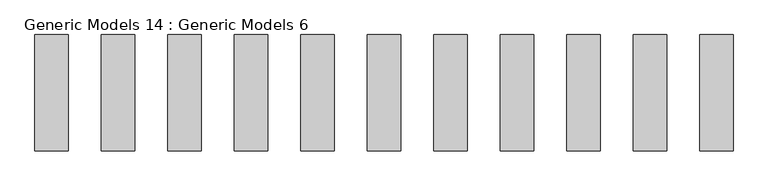
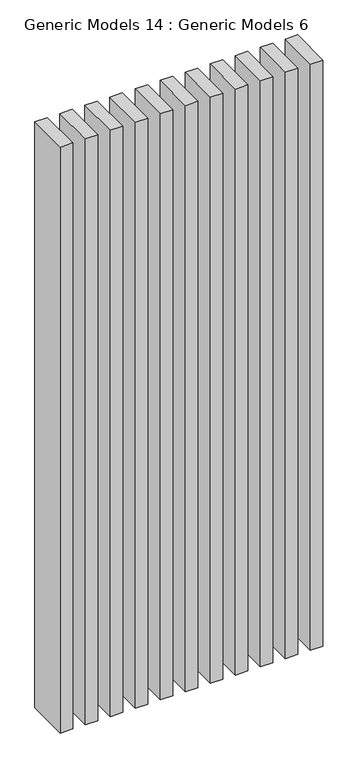
"""IFC4 building model written with IfcOpenShell, lengths in millimetres: proxy geometry, Generic Models 14 : Generic Models 6."""

from ifc_helpers import new_model, si_unit, frame, origin, place, context, project, spatial, polyline, outline, extrude, source, transform, mapped, element, save


def generic_models_14_generic_models_6_3cb9ea36(model_context):
    return source(origin(), model_context, "Body", "SweptSolid", [
        extrude(outline(polyline([(-7087.8263252, -11102.5719459), (-7138.6263252, -11102.5719459), (-7138.6263252, -10924.7719459), (-7087.8263252, -10924.7719459), (-7087.8263252, -11102.5719459)])), frame((0.0, 0.0, 3885.375135), z_axis=(0.0, 0.0, 1.0), x_axis=(1.0, 0.0, 0.0)), (0.0, 0.0, 1.0), 2515.424865),
        extrude(outline(polyline([(-6986.2263252, -11102.5719459), (-7037.0263252, -11102.5719459), (-7037.0263252, -10924.7719459), (-6986.2263252, -10924.7719459), (-6986.2263252, -11102.5719459)])), frame((0.0, 0.0, 3885.375135), z_axis=(0.0, 0.0, 1.0), x_axis=(1.0, 0.0, 0.0)), (0.0, 0.0, 1.0), 2515.424865),
        extrude(outline(polyline([(-6884.6263252, -11102.5719459), (-6935.4263252, -11102.5719459), (-6935.4263252, -10924.7719459), (-6884.6263252, -10924.7719459), (-6884.6263252, -11102.5719459)])), frame((0.0, 0.0, 3885.375135), z_axis=(0.0, 0.0, 1.0), x_axis=(1.0, 0.0, 0.0)), (0.0, 0.0, 1.0), 2515.424865),
        extrude(outline(polyline([(-6783.0263252, -11102.5719459), (-6833.8263252, -11102.5719459), (-6833.8263252, -10924.7719459), (-6783.0263252, -10924.7719459), (-6783.0263252, -11102.5719459)])), frame((0.0, 0.0, 3885.375135), z_axis=(0.0, 0.0, 1.0), x_axis=(1.0, 0.0, 0.0)), (0.0, 0.0, 1.0), 2515.424865),
        extrude(outline(polyline([(-6681.4263252, -11102.5719459), (-6732.2263252, -11102.5719459), (-6732.2263252, -10924.7719459), (-6681.4263252, -10924.7719459), (-6681.4263252, -11102.5719459)])), frame((0.0, 0.0, 3885.375135), z_axis=(0.0, 0.0, 1.0), x_axis=(1.0, 0.0, 0.0)), (0.0, 0.0, 1.0), 2515.424865),
        extrude(outline(polyline([(-6579.8263252, -11102.5719459), (-6630.6263252, -11102.5719459), (-6630.6263252, -10924.7719459), (-6579.8263252, -10924.7719459), (-6579.8263252, -11102.5719459)])), frame((0.0, 0.0, 3885.375135), z_axis=(0.0, 0.0, 1.0), x_axis=(1.0, 0.0, 0.0)), (0.0, 0.0, 1.0), 2515.424865),
        extrude(outline(polyline([(-6478.2263252, -11102.5719459), (-6529.0263252, -11102.5719459), (-6529.0263252, -10924.7719459), (-6478.2263252, -10924.7719459), (-6478.2263252, -11102.5719459)])), frame((0.0, 0.0, 3885.375135), z_axis=(0.0, 0.0, 1.0), x_axis=(1.0, 0.0, 0.0)), (0.0, 0.0, 1.0), 2515.424865),
        extrude(outline(polyline([(-6376.6263252, -11102.5719459), (-6427.4263252, -11102.5719459), (-6427.4263252, -10924.7719459), (-6376.6263252, -10924.7719459), (-6376.6263252, -11102.5719459)])), frame((0.0, 0.0, 3885.375135), z_axis=(0.0, 0.0, 1.0), x_axis=(1.0, 0.0, 0.0)), (0.0, 0.0, 1.0), 2515.424865),
        extrude(outline(polyline([(-6275.0263252, -11102.5719459), (-6325.8263252, -11102.5719459), (-6325.8263252, -10924.7719459), (-6275.0263252, -10924.7719459), (-6275.0263252, -11102.5719459)])), frame((0.0, 0.0, 3885.375135), z_axis=(0.0, 0.0, 1.0), x_axis=(1.0, 0.0, 0.0)), (0.0, 0.0, 1.0), 2515.424865),
        extrude(outline(polyline([(-6173.4263252, -11102.5719459), (-6224.2263252, -11102.5719459), (-6224.2263252, -10924.7719459), (-6173.4263252, -10924.7719459), (-6173.4263252, -11102.5719459)])), frame((0.0, 0.0, 3885.375135), z_axis=(0.0, 0.0, 1.0), x_axis=(1.0, 0.0, 0.0)), (0.0, 0.0, 1.0), 2515.424865),
        extrude(outline(polyline([(-6071.8263252, -11102.5719459), (-6122.6263252, -11102.5719459), (-6122.6263252, -10924.7719459), (-6071.8263252, -10924.7719459), (-6071.8263252, -11102.5719459)])), frame((0.0, 0.0, 3885.375135), z_axis=(0.0, 0.0, 1.0), x_axis=(1.0, 0.0, 0.0)), (0.0, 0.0, 1.0), 2515.424865),
    ])


if __name__ == "__main__":
    model = new_model("IFC4")
    model_context = context("Model", 3, world=origin())
    ifc_project = project(units=[si_unit("LENGTHUNIT", "METRE", prefix="MILLI")], contexts=[model_context])
    site = spatial("IfcSite", under=ifc_project)
    building = spatial("IfcBuilding", under=site)
    placement = place(None, origin())
    generic_models_14_generic_models_6_shape = generic_models_14_generic_models_6_3cb9ea36(model_context)
    element("IfcBuildingElementProxy", 1, Name="Generic Models 14 : Generic Models 6", ObjectType="Generic Models 14 : Generic Models 6", at=placement, inside=building, context=model_context, shape_type="MappedRepresentation", body=[
        mapped(generic_models_14_generic_models_6_shape, transform((0.0, 0.0, 0.0), x_axis=(1.0, 0.0, 0.0), y_axis=(0.0, 1.0, 0.0), z_axis=(0.0, 0.0, 1.0))),
    ])
    save(model, "model.ifc")

# Revit data of these elements
# Element 1 (IfcBuildingElementProxy, "Generic Models 14 : Generic Models 6")
#   Materials on its faces: "TEAK BROWN COLOUR"
# Materials
#   "TEAK BROWN COLOUR": class "Generic", colour RGB 120 120 120, transparency 0, Cost = 0
